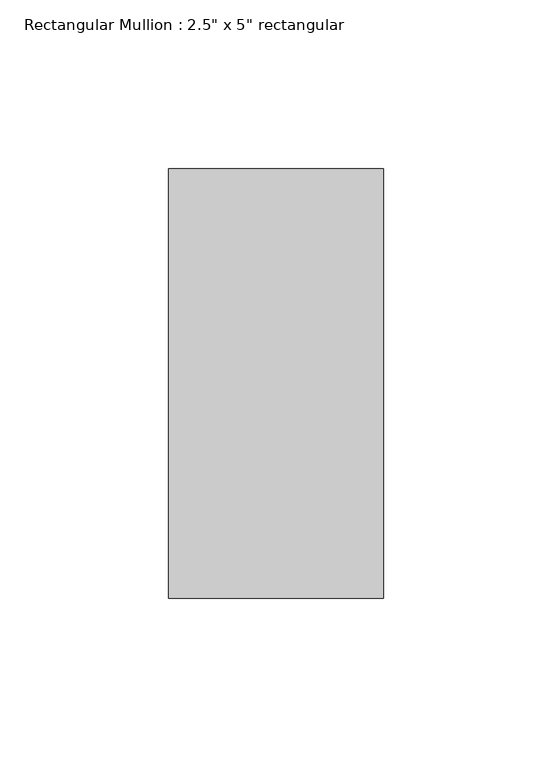
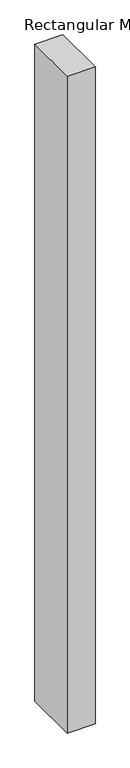
"""IFC4 building model written with IfcOpenShell, lengths in millimetres: member geometry."""

from ifc_helpers import new_model, si_unit, frame, origin, place, context, project, spatial, polyline, outline, extrude, source, transform, mapped, element, save


def member_e2840d6c(model_context):
    return source(origin(), model_context, "Body", "SweptSolid", [
        extrude(outline(polyline([(31.75, 63.5), (31.75, -63.5), (-31.75, -63.5), (-31.75, 63.5), (31.75, 63.5)])), frame((0.0, 0.0, -1580.0534505), z_axis=(0.0, 0.0, 1.0), x_axis=(1.0, 0.0, 0.0)), (0.0, 0.0, 1.0), 1580.0534505),
    ])


if __name__ == "__main__":
    model = new_model("IFC4")
    model_context = context("Model", 3, world=origin())
    ifc_project = project(units=[si_unit("LENGTHUNIT", "METRE", prefix="MILLI")], contexts=[model_context])
    site = spatial("IfcSite", under=ifc_project)
    building = spatial("IfcBuilding", under=site)
    placement = place(None, origin())
    member_shape = member_e2840d6c(model_context)
    element("IfcMember", 1, ObjectType="Rectangular Mullion : 2.5\" x 5\" rectangular", at=placement, inside=building, context=model_context, shape_type="MappedRepresentation", body=[
        mapped(member_shape, transform((0.0, 0.0, 0.0), x_axis=(1.0, 0.0, 0.0), y_axis=(0.0, 1.0, 0.0), z_axis=(0.0, 0.0, 1.0))),
    ])
    save(model, "model.ifc")

# Revit data of these elements
# Type "Rectangular Mullion : 2.5\" x 5\" rectangular"
#   built-in parameter 1007304 = 0.416667 (stored number, unit not read)
#   built-in parameter 1007301 = 0.104167 (stored number, unit not read)
#   built-in parameter 1007300 = 0.104167 (stored number, unit not read)
# Element 1 (IfcMember, "Rectangular Mullion : 2.5\" x 5\" rectangular")
#   Materials on its faces: "Aluminum"
# Materials
#   "Aluminum": class "Metal", colour RGB 247 247 247, transparency 0, Description = "Aluminum 6061", Cost = 0
